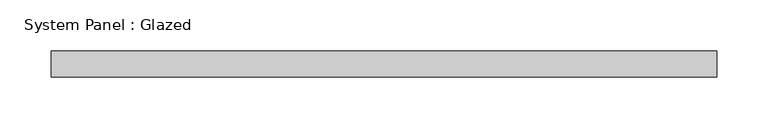
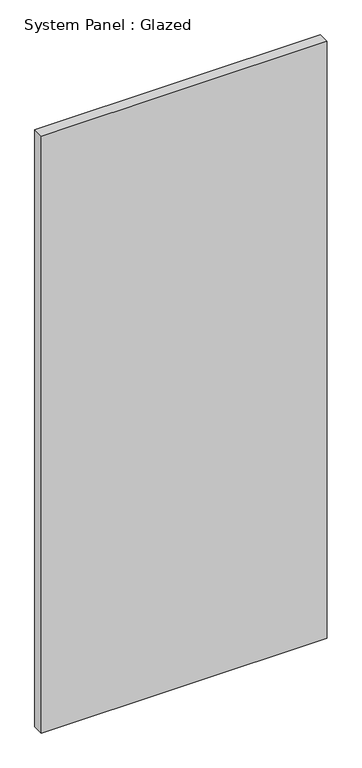
"""IFC4 building model written with IfcOpenShell, lengths in millimetres: plate geometry, System Panel : Glazed."""

from ifc_helpers import new_model, si_unit, origin, origin_with_axes, place, context, project, spatial, polyline, outline, extrude, source, transform, mapped, element, save


def system_panel_glazed_9d10e14a(model_context):
    return source(origin(), model_context, "Body", "SweptSolid", [
        extrude(outline(polyline([(323.85, 19.05), (-323.85, 19.05), (-323.85, 44.45), (323.85, 44.45), (323.85, 19.05)])), origin_with_axes(), (0.0, 0.0, 1.0), 1429.4785779),
    ])


if __name__ == "__main__":
    model = new_model("IFC4")
    model_context = context("Model", 3, world=origin())
    ifc_project = project(units=[si_unit("LENGTHUNIT", "METRE", prefix="MILLI")], contexts=[model_context])
    site = spatial("IfcSite", under=ifc_project)
    building = spatial("IfcBuilding", under=site)
    placement = place(None, origin())
    system_panel_glazed_shape = system_panel_glazed_9d10e14a(model_context)
    element("IfcPlate", 1, ObjectType="System Panel : Glazed", at=placement, inside=building, context=model_context, shape_type="MappedRepresentation", body=[
        mapped(system_panel_glazed_shape, transform((0.0, 0.0, 0.0), x_axis=(1.0, 0.0, 0.0), y_axis=(0.0, 1.0, 0.0), z_axis=(0.0, 0.0, 1.0))),
    ])
    save(model, "model.ifc")

# Revit data of these elements
# Type "System Panel : Glazed"
#   Construction Type Id = "GSP4R"
#   Analytic Construction = "1/8 in Pilkington single glazing"
#   Visual Light Transmittance = 0.9
#   Solar Heat Gain Coefficient = 0.86
#   Heat Transfer Coefficient (U) = 1.18115 BTU/(h·ft²·°F)
#   Define Thermal Properties by = 1
# Element 1 (IfcPlate, "System Panel : Glazed")
#   Materials on its faces: "Glass"
# Materials
#   "Glass": class "Glass", colour RGB 0 128 192, transparency 0.75, Description = "Soda Lime Glass", Cost = 0
